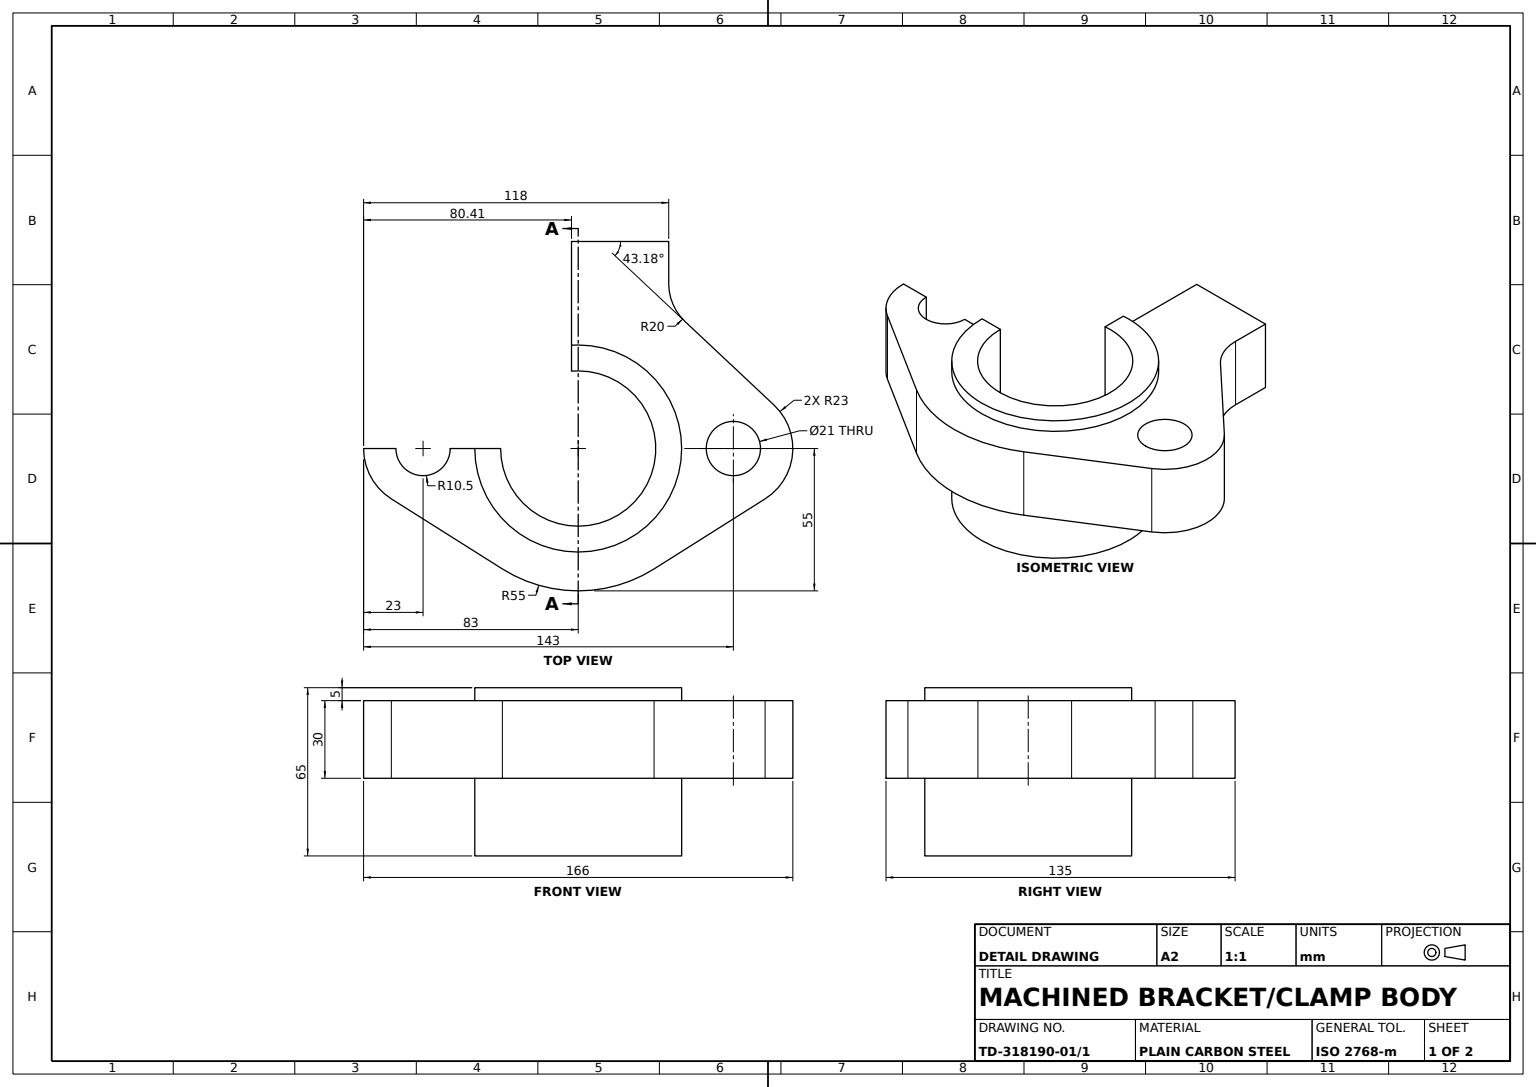
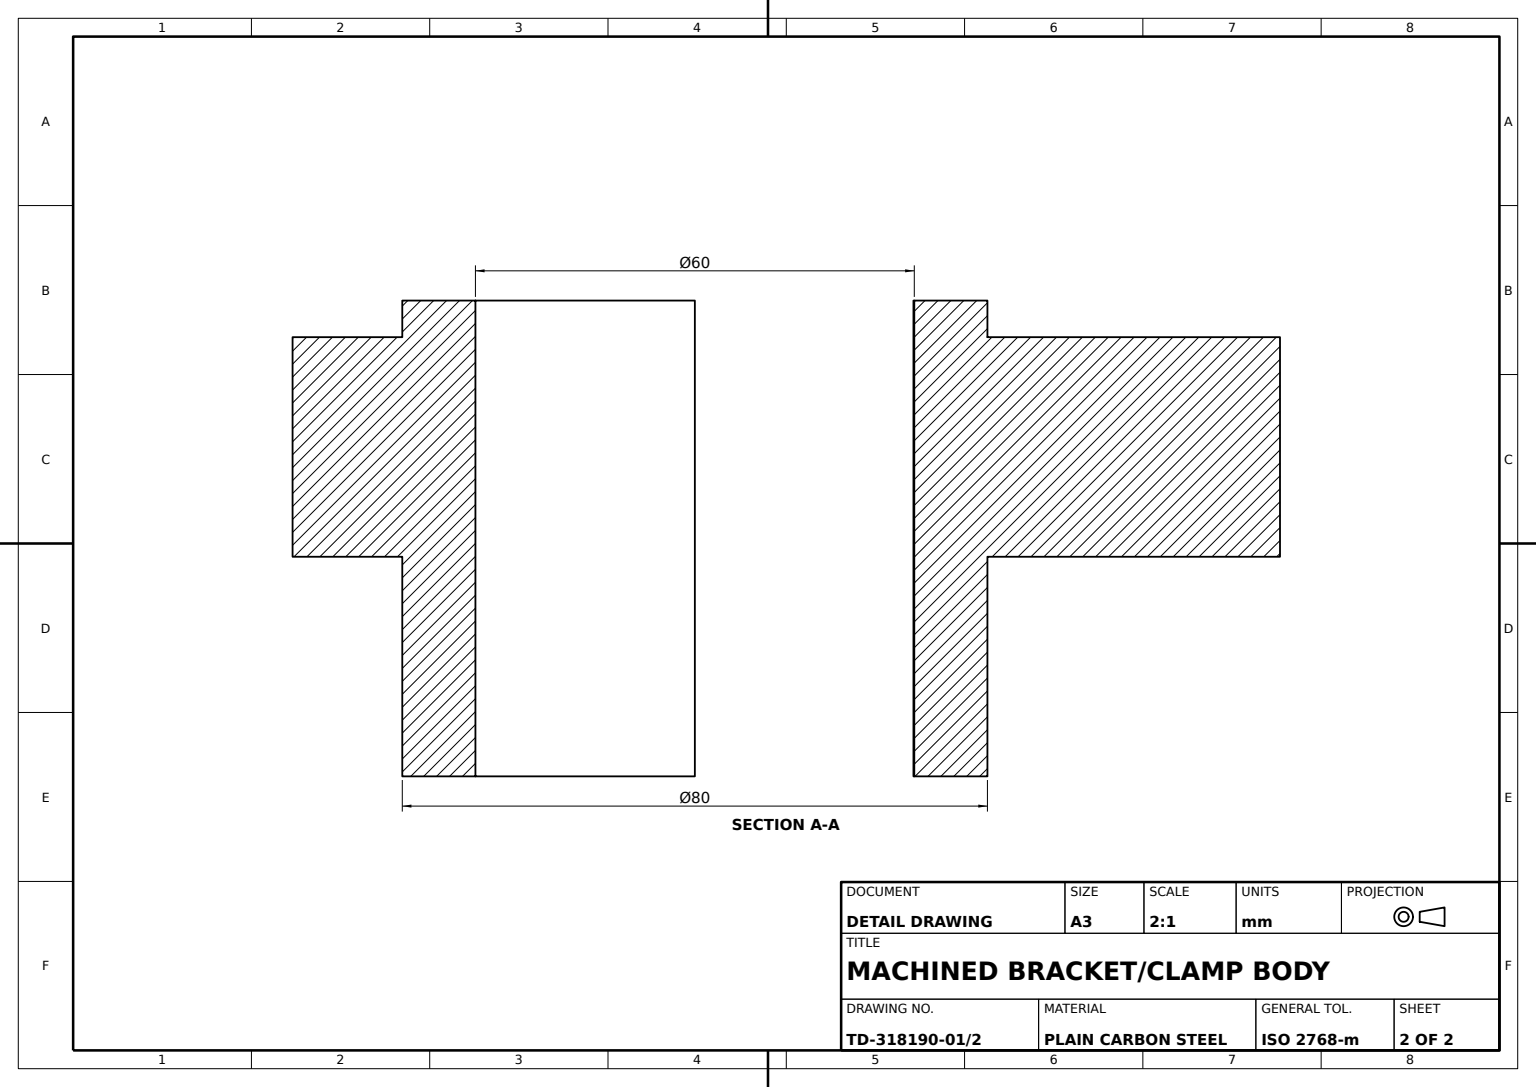
from build123d import *

# Parameters (mm, degrees)
HUB_TUBE_SKETCH_R        = 40
HUB_TUBE_SKETCH_R_2      = 30
HUB_TUBE_80_DEPTH        = 30
FLANGE_30MM_DEPTH        = 30
COLLAR_SKETCH_R          = 40
COLLAR_SKETCH_R_2        = 30
COLLAR_80_X5_DEPTH       = 5
SIDE_SLOT_CUT_DEPTH      = 135
SIDE_SLOT_CUT_DEPTH_BACK = 140
CUT_21_A_DEPTH           = 99
CUT_21_A_DEPTH_BACK      = 159
CUT_21_A_SKETCH_R        = 10.5
CUT_21_B_DEPTH           = 507
CUT_21_B_DEPTH_BACK      = 405
CUT_21_B_SKETCH_R        = 10.5


with BuildPart() as part:
    # Hub Tube Sketch → Hub Tube Ø80 (new, symmetric)
    with BuildSketch(Plane(origin=(0, 0, 0), x_dir=(1, 0, 0), z_dir=(0, 1, 0))):
        with Locations(Location((0, 0, 0), (0, 0, 270))):
            Circle(HUB_TUBE_SKETCH_R)
        with Locations(Location((0, 0, 0), (0, 0, 270))):
            Circle(HUB_TUBE_SKETCH_R_2, mode=Mode.SUBTRACT)
    extrude(amount=HUB_TUBE_80_DEPTH, both=True)

    # Flange Profile Sketch → Flange 30mm (add)
    with BuildSketch(Plane(origin=(0, 30, 0), x_dir=(1, 0, 0), z_dir=(0, 1, 0))):
        with BuildLine():
            ThreePointArc((-75.738459529, 16.772027059), (-82.895108188, -2.194087755), (-72.266666667, -19.455818895))
            Line((-72.266666667, -19.455818895), (-29.333333333, -46.524784315))
            ThreePointArc((-29.333333333, -46.524784315), (0, -55), (29.333333333, -46.524784315))
            Line((29.333333333, -46.524784315), (72.266666667, -19.455818895))
            ThreePointArc((72.266666667, -19.455818895), (82.895108188, -2.194087755), (75.738459529, 16.772027059))
            Line((75.738459529, 16.772027059), (41.314383018, 49.074737583))
            ThreePointArc((41.314383018, 49.074737583), (36.646358132, 55.712799721), (35, 63.659108939))
            Line((35, 63.659108939), (35, 80))
            Line((35, 80), (-35, 80))
            Line((-35, 80), (-35, 63.659108939))
            ThreePointArc((-35, 63.659108939), (-36.646358132, 55.712799721), (-41.314383018, 49.074737583))
            Line((-41.314383018, 49.074737583), (-75.738459529, 16.772027059))
        make_face()
        with BuildLine():
            ThreePointArc((40, 0), (-28.284271247, -28.284271247), (0, 40))
            ThreePointArc((0, 40), (28.284271247, 28.284271247), (40, 0))
        make_face(mode=Mode.SUBTRACT)
    extrude(amount=-FLANGE_30MM_DEPTH)

    # Collar Sketch → Collar Ø80 x5 (add)
    with BuildSketch(Plane(origin=(0, 30, 0), x_dir=(1, 0, 0), z_dir=(0, 1, 0))):
        with Locations(Location((0, 0, 0), (0, 0, 270))):
            Circle(COLLAR_SKETCH_R)
        with Locations(Location((0, 0, 0), (0, 0, 270))):
            Circle(COLLAR_SKETCH_R_2, mode=Mode.SUBTRACT)
    extrude(amount=COLLAR_80_X5_DEPTH)

    # Side Slot Sketch → Side Slot Cut (cut, two sides: drawn at the far end of the back side and taken through both)
    with BuildSketch(Plane.XZ.offset(-SIDE_SLOT_CUT_DEPTH_BACK)):
        Polygon((-109.161413969, 0), (-2.593057922, 0), (-2.593057922, -87.129471891), (-109.161413969, -88.900340716), align=None)
    extrude(amount=SIDE_SLOT_CUT_DEPTH + SIDE_SLOT_CUT_DEPTH_BACK, mode=Mode.SUBTRACT)

    # Cut Ø21 A Sketch → Cut Ø21 A (cut, two sides: drawn at the far end of the back side and taken through both)
    with BuildSketch(Plane.XZ.offset(-CUT_21_A_DEPTH_BACK)):
        with Locations(Location((60, 0, 0), (0, 0, 90))):
            Circle(CUT_21_A_SKETCH_R)
    extrude(amount=CUT_21_A_DEPTH + CUT_21_A_DEPTH_BACK, mode=Mode.SUBTRACT)

    # Cut Ø21 B Sketch → Cut Ø21 B (cut, two sides: drawn at the far end of the back side and taken through both)
    with BuildSketch(Plane.XZ.offset(-CUT_21_B_DEPTH_BACK)):
        with Locations((-60, 0)):
            Circle(CUT_21_B_SKETCH_R)
    extrude(amount=CUT_21_B_DEPTH + CUT_21_B_DEPTH_BACK, mode=Mode.SUBTRACT)


solid = part.part
